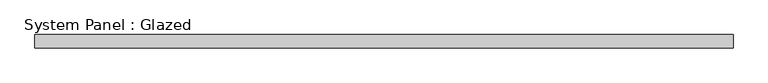
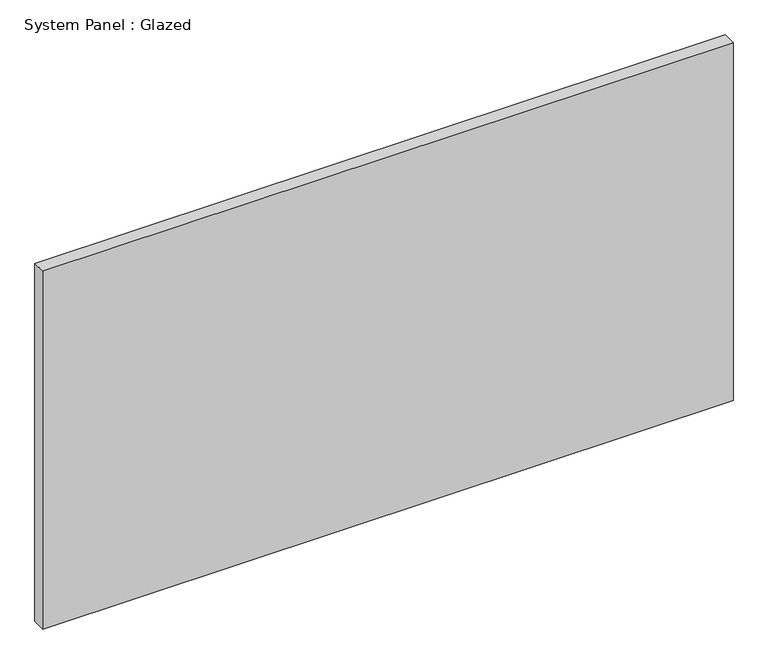
"""IFC4 building model written with IfcOpenShell, lengths in millimetres: plate geometry, System Panel : Glazed."""

from ifc_helpers import new_model, si_unit, origin, origin_with_axes, place, context, project, spatial, polyline, outline, extrude, source, transform, mapped, element, save


def system_panel_glazed_d128e385(model_context):
    return source(origin(), model_context, "Body", "SweptSolid", [
        extrude(outline(polyline([(661.32075, 19.05), (-661.32075, 19.05), (-661.32075, 44.45), (661.32075, 44.45), (661.32075, 19.05)])), origin_with_axes(), (0.0, 0.0, 1.0), 725.7415),
    ])


if __name__ == "__main__":
    model = new_model("IFC4")
    model_context = context("Model", 3, world=origin())
    ifc_project = project(units=[si_unit("LENGTHUNIT", "METRE", prefix="MILLI")], contexts=[model_context])
    site = spatial("IfcSite", under=ifc_project)
    building = spatial("IfcBuilding", under=site)
    placement = place(None, origin())
    system_panel_glazed_shape = system_panel_glazed_d128e385(model_context)
    element("IfcPlate", 1, ObjectType="System Panel : Glazed", at=placement, inside=building, context=model_context, shape_type="MappedRepresentation", body=[
        mapped(system_panel_glazed_shape, transform((0.0, 0.0, 0.0), x_axis=(1.0, 0.0, 0.0), y_axis=(0.0, 1.0, 0.0), z_axis=(0.0, 0.0, 1.0))),
    ])
    save(model, "model.ifc")

# Revit data of these elements
# Type "System Panel : Glazed"
#   Construction Type Id = "GSP4R"
#   Analytic Construction = "1/8 in Pilkington single glazing"
#   Visual Light Transmittance = 0.9
#   Solar Heat Gain Coefficient = 0.86
#   Heat Transfer Coefficient (U) = 1.18115 BTU/(h·ft²·°F)
#   Define Thermal Properties by = 1
# Element 1 (IfcPlate, "System Panel : Glazed")
#   Materials on its faces: "Glass"
# Materials
#   "Glass": class "Glass", colour RGB 0 128 192, transparency 0.75, Description = "Soda Lime Glass", Cost = 0
